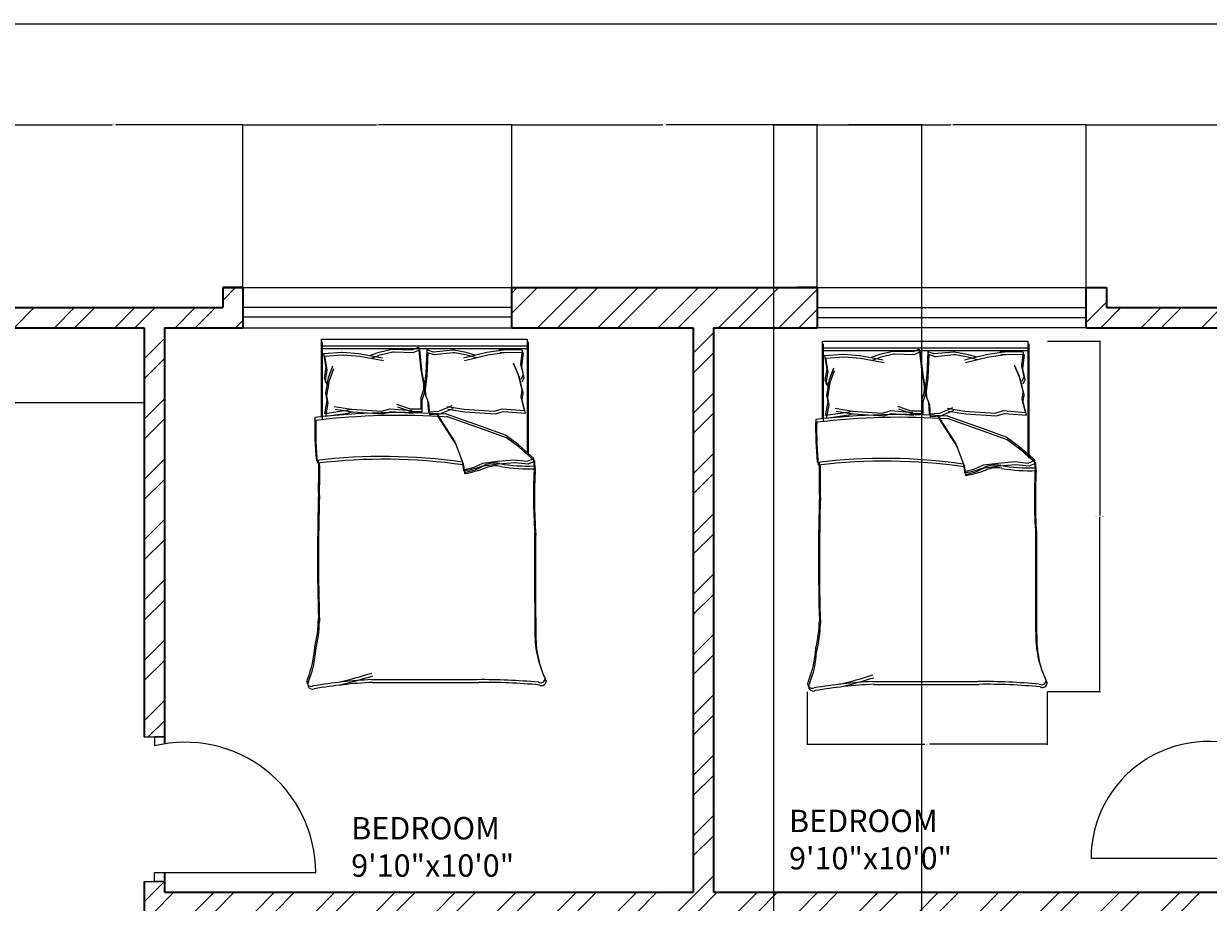
# Model space of a CAD drawing. Units: inches. Extents: x 1570 to 2186, y 1575 to 2421.
# Tile 9 of 10: x 1713 to 1978, y 2225 to 2421. Entities that reach past the tile are written whole.
import ezdxf

# ---------------------------------------------------------------- set-up
doc = ezdxf.new("R2010")
doc.units = ezdxf.units.IN
for name, color, linetype, lineweight in [('A-ANNO-DIMS', 2, 'Continuous', 18), ('A-ANNO-TTLB', 7, 'Continuous', 25), ('A-AREA-IDEN', 7, 'Continuous', 18), ('A-DOOR', 201, 'Continuous', 18), ('A-FLOR-CASE', 7, 'Continuous', 18), ('A-FURN', 8, 'Continuous', 13), ('A-GLAZ', 150, 'Continuous', 18), ('A-WALL', 7, 'Continuous', 35), ('A-WALL-PATT', 252, 'Continuous', 13)]:
    doc.layers.add(name, color=color, linetype=linetype, lineweight=lineweight)
doc.styles.get("Standard").update_dxf_attribs({"font": 'arial.ttf'})
doc.dimstyles.get("Standard").update_dxf_attribs({"dimtxt": 0.18, "dimasz": 0.18, "dimexe": 0.18, "dimexo": 0.0625, "dimgap": 0.09, "dimtad": 0, "dimtih": 1, "dimtoh": 1, "dimdec": 4, "dimzin": 0, "dimdsep": 46, "dimtxsty": 'Standard', "dimcen": 0.09, "dimadec": 0, "dimazin": 0, "dimtfac": 1, "dimtdec": 4, "dimtofl": 0, "dimtmove": 0, "dimatfit": 3, "dimfxl": 1, "dimtolj": 1, "dimtzin": 0, "dimarcsym": 0})

# ---------------------------------------------------------------- blocks, each defined once
blk = doc.blocks.new('BED-DOUBLE')
for p, q in [((3.33, 60.74), (3.33, 78.1)), ((3.33, 60.74), (3.33, 78.1)), ((3.33, 78.1), (49.16, 78.1)), ((3.55, 60.12), (3.55, 77.49)), ((3.55, 60.12), (3.55, 77.49)), ((49.16, 78.1), (49.16, 52.58)), ((49.16, 78.1), (49.16, 52.58)), ((49.38, 77.49), (49.38, 51.97)), ((49.38, 77.49), (49.38, 51.97)), ((3.33, 76.63), (49.16, 76.63)), ((3.33, 76.63), (49.16, 76.63)), ((3.55, 76.02), (49.38, 76.02)), ((3.55, 76.02), (49.38, 76.02)), ((3.74, 74.9), (7.84, 75.22)), ((3.74, 74.9), (7.84, 75.22)), ((3.74, 74.92), (4.29, 71.87)), ((3.74, 74.92), (4.29, 71.87)), ((3.95, 74.31), (4.51, 71.26)), ((3.95, 74.31), (4.51, 71.26)), ((3.96, 74.29), (8.06, 74.6)), ((3.96, 74.29), (8.06, 74.6)), ((7.84, 75.22), (7.95, 75.2)), ((7.84, 75.22), (7.95, 75.2)), ((7.95, 75.2), (11.61, 74.92)), ((7.95, 75.2), (11.61, 74.92)), ((8.06, 74.6), (8.16, 74.59)), ((8.06, 74.6), (8.16, 74.59)), ((8.16, 74.59), (11.83, 74.31)), ((8.16, 74.59), (11.83, 74.31)), ((11.61, 74.92), (16.88, 73.95)), ((11.61, 74.92), (16.88, 73.95)), ((11.83, 74.31), (17.1, 73.34)), ((11.83, 74.31), (17.1, 73.34)), ((14.25, 74.51), (16.19, 75.2)), ((14.25, 74.51), (16.19, 75.2)), ((14.46, 73.89), (16.41, 74.59)), ((14.47, 73.89), (16.41, 74.59)), ((16.19, 75.2), (18.96, 75.89)), ((16.19, 75.2), (18.96, 75.89)), ((16.41, 74.59), (19.18, 75.28)), ((16.41, 74.59), (19.18, 75.28)), ((18.96, 75.89), (19.27, 75.89)), ((18.96, 75.89), (19.27, 75.89)), ((19.18, 75.28), (19.49, 75.28)), ((19.18, 75.28), (19.49, 75.28)), ((19.27, 75.89), (23.53, 75.76)), ((19.27, 75.89), (23.53, 75.76)), ((19.49, 75.28), (23.75, 75.14)), ((19.49, 75.28), (23.75, 75.14)), ((23.53, 75.76), (24.92, 76.31)), ((23.53, 75.76), (24.92, 76.31)), ((23.75, 75.14), (25.14, 75.7)), ((23.75, 75.14), (25.14, 75.7)), ((24.92, 76.31), (25.47, 71.18)), ((24.92, 76.31), (25.47, 71.18)), ((25.14, 75.7), (25.69, 70.57)), ((25.14, 75.7), (25.69, 70.57)), ((26.83, 75.71), (26.6, 70.56)), ((26.83, 75.71), (26.6, 70.56)), ((27.05, 75.1), (26.82, 69.95)), ((27.05, 75.1), (26.82, 69.95)), ((28.25, 75.25), (26.83, 75.71)), ((28.25, 75.25), (26.83, 75.71)), ((28.47, 74.63), (27.05, 75.1)), ((28.47, 74.63), (27.05, 75.1)), ((32.49, 75.65), (28.25, 75.25)), ((32.49, 75.65), (28.25, 75.25)), ((32.71, 75.04), (28.47, 74.63)), ((32.71, 75.04), (28.47, 74.63)), ((32.8, 75.67), (32.49, 75.65)), ((32.8, 75.67), (32.49, 75.65)), ((33.02, 75.06), (32.71, 75.04)), ((33.02, 75.06), (32.71, 75.04)), ((35.61, 75.15), (32.8, 75.67)), ((35.61, 75.15), (32.8, 75.67)), ((35.83, 74.54), (33.02, 75.06)), ((35.83, 74.54), (33.02, 75.06)), ((40.2, 75.16), (35, 73.86)), ((40.2, 75.16), (35, 73.86)), ((40.42, 74.55), (35.22, 73.25)), ((40.41, 74.55), (35.22, 73.25)), ((37.59, 74.58), (35.61, 75.15)), ((37.59, 74.58), (35.61, 75.15)), ((37.81, 73.97), (35.83, 74.54)), ((37.81, 73.97), (35.83, 74.54)), ((43.84, 75.67), (40.2, 75.16)), ((43.84, 75.67), (40.2, 75.16)), ((44.06, 75.05), (40.41, 74.55)), ((44.06, 75.05), (40.42, 74.55)), ((48.06, 75.65), (42.88, 75.74)), ((42.88, 75.74), (43.84, 75.67)), ((48.06, 75.65), (42.88, 75.74)), ((42.88, 75.74), (43.84, 75.67)), ((48.28, 75.04), (43.1, 75.13)), ((43.1, 75.13), (44.06, 75.05)), ((48.28, 75.04), (43.1, 75.13)), ((43.1, 75.13), (44.06, 75.05)), ((48.06, 75.65), (47.69, 72.57)), ((48.06, 75.65), (47.69, 72.57)), ((48.28, 75.04), (47.91, 71.96)), ((48.28, 75.04), (47.91, 71.96)), ((4.29, 71.87), (3.87, 69.38)), ((4.29, 71.87), (3.87, 69.38)), ((4.84, 69.52), (5.81, 72.15)), ((4.84, 69.52), (5.81, 72.15)), ((5.06, 68.9), (6.03, 71.54)), ((5.06, 68.9), (6.03, 71.54)), ((47.29, 70.18), (46.15, 72.75)), ((47.29, 70.18), (46.16, 72.75)), ((47.51, 69.57), (46.37, 72.14)), ((47.51, 69.57), (46.37, 72.14)), ((47.69, 72.57), (48.27, 70.11)), ((47.69, 72.57), (48.26, 70.11)), ((47.91, 71.96), (48.48, 69.49)), ((47.91, 71.96), (48.48, 69.49)), ((3.87, 69.38), (4.43, 68.41)), ((3.87, 69.38), (4.43, 68.41)), ((4.51, 71.26), (4.09, 68.76)), ((4.51, 71.26), (4.09, 68.76)), ((4.09, 68.76), (4.65, 67.79)), ((4.09, 68.76), (4.65, 67.79)), ((4.29, 66.05), (4.84, 69.52)), ((4.29, 66.05), (4.84, 69.52)), ((4.51, 65.44), (5.06, 68.9)), ((4.51, 65.44), (5.06, 68.9)), ((25.47, 71.18), (26.03, 68.13)), ((25.47, 71.18), (26.03, 68.13)), ((25.69, 70.57), (26.25, 67.52)), ((25.69, 70.57), (26.25, 67.52)), ((26.6, 70.56), (26.23, 67.48)), ((26.6, 70.56), (26.23, 67.48)), ((26.82, 69.95), (26.45, 66.87)), ((26.82, 69.95), (26.45, 66.87)), ((48.06, 66.76), (47.29, 70.18)), ((48.06, 66.76), (47.29, 70.18)), ((48.28, 66.15), (47.51, 69.57)), ((48.28, 66.15), (47.51, 69.57)), ((48.27, 70.11), (47.77, 69.1)), ((48.26, 70.11), (47.77, 69.1)), ((48.48, 69.49), (47.99, 68.49)), ((48.48, 69.49), (47.99, 68.49)), ((26.03, 66.88), (25.47, 65.08)), ((26.03, 66.88), (25.47, 65.08)), ((26.25, 66.27), (25.69, 64.47)), ((26.25, 66.27), (25.69, 64.47)), ((26.03, 68.13), (26.03, 66.88)), ((26.03, 68.13), (26.03, 66.88)), ((26.23, 67.48), (26.31, 66.23)), ((26.23, 67.48), (26.31, 66.23)), ((26.25, 67.52), (26.25, 66.27)), ((26.25, 67.52), (26.25, 66.27)), ((26.31, 66.23), (26.98, 64.47)), ((26.31, 66.23), (26.98, 64.47)), ((26.45, 66.87), (26.53, 65.62)), ((26.45, 66.87), (26.53, 65.62)), ((47.88, 65.22), (48.06, 66.76)), ((47.88, 65.22), (48.06, 66.76)), ((48.09, 64.61), (48.28, 66.15)), ((48.1, 64.61), (48.28, 66.15)), ((4.01, 61.47), (4.57, 64.52)), ((4.01, 61.47), (4.57, 64.52)), ((4.23, 60.86), (4.79, 63.91)), ((4.23, 60.86), (4.79, 63.91)), ((4.57, 64.52), (4.29, 66.05)), ((4.57, 64.52), (4.29, 66.05)), ((4.79, 63.91), (4.51, 65.44)), ((4.79, 63.91), (4.51, 65.44)), ((23.12, 62.51), (20.1, 63.55)), ((23.12, 62.51), (20.1, 63.55)), ((25.47, 65.08), (25.47, 62.51)), ((25.47, 65.08), (25.47, 62.51)), ((25.69, 64.47), (25.69, 61.89)), ((25.69, 64.47), (25.69, 61.89)), ((26.53, 65.62), (27.2, 63.86)), ((26.53, 65.62), (27.2, 63.86)), ((26.98, 64.47), (27.14, 61.9)), ((26.98, 64.47), (27.14, 61.9)), ((27.2, 63.86), (27.36, 61.29)), ((27.2, 63.86), (27.36, 61.29)), ((48.62, 62.21), (47.88, 65.22)), ((48.62, 62.21), (47.88, 65.22)), ((48.84, 61.6), (48.09, 64.61)), ((48.84, 61.6), (48.1, 64.61)), ((8.9, 62.17), (4.01, 61.47)), ((8.9, 62.17), (4.01, 61.47)), ((9.12, 61.55), (4.23, 60.86)), ((9.12, 61.55), (4.23, 60.86)), ((6.12, 63.12), (9.99, 62.48)), ((6.12, 63.12), (9.99, 62.48)), ((6.34, 62.5), (10.21, 61.86)), ((6.34, 62.5), (10.21, 61.86)), ((9.99, 62.48), (8.9, 62.17)), ((9.99, 62.48), (8.9, 62.17)), ((10.21, 61.86), (9.12, 61.55)), ((10.21, 61.86), (9.12, 61.55)), ((9.99, 62.48), (16.71, 62.06)), ((9.99, 62.48), (16.71, 62.06)), ((10.21, 61.86), (16.93, 61.45)), ((10.21, 61.86), (16.93, 61.45)), ((16.71, 62.06), (18.59, 62.6)), ((16.71, 62.06), (18.59, 62.6)), ((16.93, 61.45), (18.81, 61.98)), ((16.93, 61.45), (18.81, 61.98)), ((18.59, 62.6), (23.51, 62.21)), ((18.59, 62.6), (23.51, 62.21)), ((18.81, 61.98), (23.73, 61.6)), ((18.81, 61.98), (23.73, 61.6)), ((23.33, 61.89), (20.32, 62.94)), ((23.33, 61.89), (20.32, 62.94)), ((25.47, 62.51), (23.12, 62.51)), ((25.47, 62.51), (23.12, 62.51)), ((25.69, 61.89), (23.33, 61.89)), ((25.69, 61.89), (23.33, 61.89)), ((27.14, 61.9), (29.49, 62.05)), ((27.14, 61.9), (29.49, 62.05)), ((27.36, 61.29), (29.71, 61.44)), ((27.36, 61.29), (29.71, 61.44)), ((29.02, 61.43), (33.04, 55.21)), ((29.02, 61.43), (33.04, 55.21)), ((29.24, 60.82), (33.26, 54.59)), ((29.24, 60.82), (33.26, 54.59)), ((29.49, 62.05), (32.43, 63.28)), ((29.49, 62.05), (32.43, 63.28)), ((29.71, 61.44), (32.65, 62.67)), ((29.71, 61.44), (32.65, 62.67)), ((38.98, 58.62), (30.98, 61.43)), ((38.98, 58.62), (30.98, 61.43)), ((39.2, 58.01), (31.2, 60.82)), ((39.2, 58.01), (31.2, 60.82)), ((31.23, 63.12), (35.1, 62.48)), ((31.23, 63.12), (35.1, 62.48)), ((31.45, 62.5), (35.31, 61.86)), ((31.45, 62.5), (35.31, 61.86)), ((35.1, 62.48), (41.82, 62.06)), ((35.1, 62.48), (41.82, 62.06)), ((35.31, 61.86), (42.04, 61.45)), ((35.31, 61.86), (42.04, 61.45)), ((41.82, 62.06), (43.7, 62.6)), ((41.82, 62.06), (43.7, 62.6)), ((42.04, 61.45), (43.92, 61.98)), ((42.04, 61.45), (43.92, 61.98)), ((43.7, 62.6), (48.62, 62.21)), ((43.7, 62.6), (48.62, 62.21)), ((43.92, 61.98), (48.84, 61.6)), ((43.92, 61.98), (48.84, 61.6)), ((44.32, 56.69), (38.98, 58.62)), ((44.32, 56.69), (38.98, 58.62)), ((44.54, 56.08), (39.2, 58.01)), ((44.54, 56.08), (39.2, 58.01)), ((47.15, 54.61), (44.32, 56.69)), ((47.15, 54.61), (44.32, 56.69)), ((47.37, 54), (44.54, 56.08)), ((47.37, 54), (44.54, 56.08)), ((33.04, 55.21), (34.67, 50.9)), ((33.04, 55.21), (34.67, 50.9)), ((33.26, 54.59), (34.89, 50.29)), ((33.26, 54.59), (34.89, 50.29)), ((50.7, 51.5), (47.15, 54.61)), ((50.7, 51.5), (47.15, 54.61)), ((50.92, 50.88), (47.37, 54)), ((50.92, 50.88), (47.37, 54)), ((34.67, 50.9), (34.97, 48.97)), ((34.67, 50.9), (34.97, 48.97)), ((34.89, 50.29), (35.19, 48.36)), ((34.89, 50.29), (35.19, 48.36)), ((37.34, 49.57), (39.27, 50.46)), ((37.34, 49.57), (39.27, 50.46)), ((39.27, 50.46), (42.54, 50.9)), ((39.27, 50.46), (42.54, 50.9)), ((39.49, 49.84), (42.76, 50.29)), ((39.49, 49.84), (42.76, 50.29)), ((42.54, 50.9), (46.26, 51.2)), ((42.54, 50.9), (46.26, 51.2)), ((42.76, 50.29), (46.47, 50.59)), ((42.76, 50.29), (46.47, 50.59)), ((46.26, 51.2), (49.23, 50.9)), ((46.26, 51.2), (49.23, 50.9)), ((46.47, 50.59), (49.45, 50.29)), ((46.47, 50.59), (49.44, 50.29)), ((49.23, 50.9), (50.7, 51.5)), ((49.23, 50.9), (50.7, 51.5)), ((49.44, 50.29), (50.92, 50.88)), ((49.45, 50.29), (50.92, 50.88)), ((50.78, 49.82), (50.7, 51.5, 3.71)), ((50.78, 49.82), (50.7, 51.5, 3.71)), ((51, 49.21), (50.92, 50.88, 3.71)), ((51, 49.21), (50.92, 50.88, 3.71)), ((34.97, 48.97), (37.34, 49.57)), ((34.97, 48.97), (37.34, 49.57)), ((35.19, 48.36), (37.56, 48.95)), ((35.19, 48.36), (37.56, 48.95)), ((37.56, 48.95), (39.49, 49.84)), ((37.56, 48.95), (39.49, 49.84)), ((14.45, 2.11), (38.05, 2.11)), ((14.45, 2.11), (38.05, 2.11)), ((14.66, 1.49), (38.27, 1.49)), ((14.67, 1.49), (38.27, 1.49))]:
    blk.add_line(p, q)
for centre, radius, start, end in [((20.48, -96.48), 158.2, 86.0865, 96.7821), ((20.48, -96.48), 158.2, 86.0865, 96.7821), ((20.7, -97.1), 158.2, 86.0865, 96.7821), ((20.7, -97.1), 158.2, 86.0865, 96.7821), ((81.67, 58.83), 79.89, 178.7218, 185.604), ((81.67, 58.83), 79.89, 178.7218, 185.604), ((81.89, 58.22), 79.89, 178.7218, 185.604), ((81.89, 58.22), 79.89, 178.7218, 185.604), ((17.03, -71.8), 123.73, 81.7845, 96.9006), ((17.03, -71.8), 123.73, 81.7845, 96.9006), ((17.25, -72.42), 123.73, 81.7845, 96.9006), ((17.25, -72.42), 123.73, 81.7845, 96.9006), ((-160.45, 48.21), 163.13, 358.4762, 1.0082), ((-160.45, 48.21), 163.13, 358.4762, 1.0082), ((-160.23, 47.59), 163.13, 358.4762, 1.0082), ((-160.23, 47.59), 163.13, 358.4762, 1.0082), ((41.95, 44.48), 5.97, 78.6608, 113.7384), ((41.95, 44.48), 5.97, 78.6608, 113.7384), ((49.22, 84.49), 34.7, 259.8763, 272.5657), ((49.22, 84.49), 34.7, 259.8763, 272.5657), ((35.13, 48.91), 0.177, 160.2464, 271.1377), ((35.13, 48.91), 0.177, 160.2464, 271.1377), ((29.88, 76.68), 28.44, 280.6617, 289.8806), ((29.88, 76.68), 28.44, 280.6617, 289.8806), ((35.35, 48.3), 0.177, 160.2464, 271.1377), ((35.35, 48.3), 0.177, 160.2464, 271.1377), ((30.1, 76.07), 28.44, 280.6617, 289.8806), ((30.1, 76.07), 28.44, 280.6617, 289.8806), ((42.17, 43.86), 5.97, 78.6608, 113.7384), ((42.17, 43.86), 5.97, 78.6608, 113.7384), ((49.44, 83.87), 34.7, 259.8763, 272.5657), ((49.44, 83.87), 34.7, 259.8763, 272.5657), ((174.79, 43.28), 124.19, 176.9791, 183.8365), ((174.79, 43.28), 124.19, 176.9791, 183.8365), ((175.01, 42.66), 124.19, 176.9791, 183.8365), ((175.01, 42.66), 124.19, 176.9791, 183.8365), ((464.94, 29.56), 462.53, 178.2277, 181.7185), ((464.94, 29.56), 462.53, 178.2277, 181.7185), ((465.16, 28.95), 462.53, 178.2277, 181.7185), ((465.16, 28.95), 462.53, 178.2277, 181.7185), ((-4323.86, 13.06), 4374.8, 0.00217, 0.28689), ((-4323.86, 13.06), 4374.8, 0.00217, 0.28689), ((-4323.64, 12.45), 4374.8, 0.00217, 0.28689), ((-4323.64, 12.45), 4374.8, 0.00217, 0.28689), ((-25.8, 16.23), 28.42, 346.0648, 358.9113), ((-25.8, 16.23), 28.42, 346.0648, 358.9113), ((-25.58, 15.62), 28.42, 346.0648, 358.9113), ((-25.58, 15.62), 28.42, 346.0648, 358.9113), ((73.03, 12.25), 22.12, 177.4714, 206.4681), ((73.03, 12.25), 22.12, 177.4714, 206.4681), ((73.25, 11.64), 22.12, 177.4714, 206.4681), ((73.25, 11.64), 22.12, 177.4714, 206.4681), ((-20.77, 10.71), 22.6, 337.9751, 356.652), ((-20.77, 10.71), 22.6, 337.9751, 356.652), ((-20.55, 10.1), 22.6, 337.9751, 356.652), ((-20.55, 10.1), 22.6, 337.9751, 356.652), ((-16.52, 100.84), 102.09, 283.3832, 287.7053), ((-16.52, 100.84), 102.09, 283.3832, 287.7053), ((-16.3, 100.23), 102.09, 283.3832, 287.7053), ((-16.3, 100.23), 102.09, 283.3832, 287.7053), ((1.04, 1.65), 1.04, 146.1736, 293.4781), ((1.04, 1.65), 1.04, 146.1736, 293.4781), ((1.26, 1.04), 1.04, 146.1736, 293.4781), ((1.26, 1.04), 1.04, 146.1736, 293.4781), ((20.55, -114.5), 116.77, 92.9958, 99.4091), ((20.55, -114.5), 116.77, 92.9958, 99.4091), ((20.77, -115.11), 116.77, 92.9958, 99.4091), ((20.77, -115.11), 116.77, 92.9958, 99.4091), ((39.46, -125.47), 127.58, 84.4998, 90.6351), ((39.46, -125.47), 127.58, 84.4998, 90.6351), ((39.68, -126.08), 127.58, 84.4998, 90.6351), ((39.68, -126.08), 127.58, 84.4998, 90.6351), ((52.18, 2.47), 1.06, 242.6588, 356.02), ((52.18, 2.47), 1.06, 242.6588, 356.02), ((52.4, 1.85), 1.06, 242.6588, 356.02), ((52.4, 1.85), 1.06, 242.6588, 356.02)]:
    blk.add_arc(centre, radius, start, end)
blk = doc.blocks.new('*D14')
at = {"layer": 'A-ANNO-DIMS', "color": 0, "lineweight": -2, "transparency": 16777216}
for p, q in [((1941.63, 2350.17), (1953.47, 2350.17)), ((1953.29, 2349.99), (1953.29, 2311.25)), ((1953.29, 2272.15), (1953.29, 2310.89)), ((1941.63, 2271.97), (1953.47, 2271.97))]:
    blk.add_line(p, q, dxfattribs=at)
at = {"layer": 'A-ANNO-DIMS', "color": 0, "transparency": 16777216}
for points in [[(1953.26, 2349.99), (1953.32, 2349.99), (1953.29, 2350.17)], [(1953.26, 2272.15), (1953.32, 2272.15), (1953.29, 2271.97)]]:
    blk.add_solid(points, dxfattribs=at)
at = {"layer": 'Defpoints', "color": 0, "transparency": 16777216}
for p in [(1941.56, 2350.17), (1953.29, 2350.17), (1941.56, 2271.97)]:
    blk.add_point(p, dxfattribs=at)
at = {"layer": 'A-ANNO-DIMS', "color": 0, "transparency": 16777216, "insert": (1953.29, 2311.07), "char_height": 0.18, "attachment_point": 5}
blk.add_mtext('\\A1;DOUBLE BED 78 TYP.', dxfattribs=at)
blk = doc.blocks.new('*D15')
at = {"layer": 'A-ANNO-DIMS', "color": 0, "lineweight": -2, "transparency": 16777216}
for p, q in [((1888.03, 2271.91), (1888.03, 2260.06)), ((1941.56, 2271.91), (1941.56, 2260.06)), ((1888.21, 2260.24), (1914.27, 2260.24)), ((1941.38, 2260.24), (1915.32, 2260.24))]:
    blk.add_line(p, q, dxfattribs=at)
at = {"layer": 'A-ANNO-DIMS', "color": 0, "transparency": 16777216}
for points in [[(1888.21, 2260.27), (1888.21, 2260.21), (1888.03, 2260.24)], [(1941.38, 2260.27), (1941.38, 2260.21), (1941.56, 2260.24)]]:
    blk.add_solid(points, dxfattribs=at)
at = {"layer": 'Defpoints', "color": 0, "transparency": 16777216}
for p in [(1888.03, 2271.97), (1941.56, 2271.97), (1941.56, 2260.24)]:
    blk.add_point(p, dxfattribs=at)
at = {"layer": 'A-ANNO-DIMS', "color": 0, "transparency": 16777216, "insert": (1914.8, 2260.24), "char_height": 0.18, "attachment_point": 5}
blk.add_mtext('\\A1;54 TYP.', dxfattribs=at)
blk = doc.blocks.new('*D24')
at = {"layer": 'A-ANNO-DIMS', "color": 0, "lineweight": -2, "transparency": 16777216}
for p, q in [((1704.62, 2362.21), (1704.62, 2398.63)), ((1704.8, 2398.45), (1732.96, 2398.45)), ((1761.92, 2398.45), (1733.75, 2398.45)), ((1762.1, 2362.21), (1762.1, 2398.63))]:
    blk.add_line(p, q, dxfattribs=at)
at = {"layer": 'A-ANNO-DIMS', "color": 0, "transparency": 16777216}
for points in [[(1704.8, 2398.48), (1704.8, 2398.42), (1704.62, 2398.45)], [(1761.92, 2398.48), (1761.92, 2398.42), (1762.1, 2398.45)]]:
    blk.add_solid(points, dxfattribs=at)
at = {"layer": 'Defpoints', "color": 0, "transparency": 16777216}
for p in [(1762.1, 2398.45), (1704.62, 2362.15), (1762.1, 2362.15)]:
    blk.add_point(p, dxfattribs=at)
at = {"layer": 'A-ANNO-DIMS', "color": 0, "transparency": 16777216, "insert": (1733.36, 2398.45), "char_height": 0.18, "attachment_point": 5}
blk.add_mtext('\\A1;57.48', dxfattribs=at)
blk = doc.blocks.new('*D25')
at = {"layer": 'A-ANNO-DIMS', "color": 0, "lineweight": -2, "transparency": 16777216}
for p, q in [((1762.1, 2362.21), (1762.1, 2398.63)), ((1762.28, 2398.45), (1791.88, 2398.45)), ((1821.92, 2398.45), (1792.32, 2398.45)), ((1822.1, 2362.21), (1822.1, 2398.63))]:
    blk.add_line(p, q, dxfattribs=at)
at = {"layer": 'A-ANNO-DIMS', "color": 0, "transparency": 16777216}
for points in [[(1762.28, 2398.48), (1762.28, 2398.42), (1762.1, 2398.45)], [(1821.92, 2398.48), (1821.92, 2398.42), (1822.1, 2398.45)]]:
    blk.add_solid(points, dxfattribs=at)
at = {"layer": 'Defpoints', "color": 0, "transparency": 16777216}
for p in [(1822.1, 2398.45), (1762.1, 2362.15), (1822.1, 2362.15)]:
    blk.add_point(p, dxfattribs=at)
at = {"layer": 'A-ANNO-DIMS', "color": 0, "transparency": 16777216, "insert": (1792.1, 2398.45), "char_height": 0.18, "attachment_point": 5}
blk.add_mtext('\\A1;60', dxfattribs=at)
blk = doc.blocks.new('*D26')
at = {"layer": 'A-ANNO-DIMS', "color": 0, "lineweight": -2, "transparency": 16777216}
for p, q in [((1822.1, 2362.21), (1822.1, 2398.63)), ((1822.28, 2398.45), (1855.78, 2398.45)), ((1890.08, 2398.45), (1856.57, 2398.45)), ((1890.26, 2362.21), (1890.26, 2398.63))]:
    blk.add_line(p, q, dxfattribs=at)
at = {"layer": 'A-ANNO-DIMS', "color": 0, "transparency": 16777216}
for points in [[(1822.28, 2398.48), (1822.28, 2398.42), (1822.1, 2398.45)], [(1890.08, 2398.48), (1890.08, 2398.42), (1890.26, 2398.45)]]:
    blk.add_solid(points, dxfattribs=at)
at = {"layer": 'Defpoints', "color": 0, "transparency": 16777216}
for p in [(1890.26, 2398.45), (1822.1, 2362.15), (1890.26, 2362.15)]:
    blk.add_point(p, dxfattribs=at)
at = {"layer": 'A-ANNO-DIMS', "color": 0, "transparency": 16777216, "insert": (1856.18, 2398.45), "char_height": 0.18, "attachment_point": 5}
blk.add_mtext('\\A1;68.16', dxfattribs=at)
blk = doc.blocks.new('*D27')
at = {"layer": 'A-ANNO-DIMS', "color": 0, "lineweight": -2, "transparency": 16777216}
for p, q in [((1890.26, 2362.21), (1890.26, 2398.63)), ((1890.44, 2398.45), (1920.04, 2398.45)), ((1950.08, 2398.45), (1920.48, 2398.45)), ((1950.26, 2362.21), (1950.26, 2398.63))]:
    blk.add_line(p, q, dxfattribs=at)
at = {"layer": 'A-ANNO-DIMS', "color": 0, "transparency": 16777216}
for points in [[(1890.44, 2398.48), (1890.44, 2398.42), (1890.26, 2398.45)], [(1950.08, 2398.48), (1950.08, 2398.42), (1950.26, 2398.45)]]:
    blk.add_solid(points, dxfattribs=at)
at = {"layer": 'Defpoints', "color": 0, "transparency": 16777216}
for p in [(1950.26, 2398.45), (1890.26, 2362.15), (1950.26, 2362.15)]:
    blk.add_point(p, dxfattribs=at)
at = {"layer": 'A-ANNO-DIMS', "color": 0, "transparency": 16777216, "insert": (1920.26, 2398.45), "char_height": 0.18, "attachment_point": 5}
blk.add_mtext('\\A1;60', dxfattribs=at)
blk = doc.blocks.new('*D28')
at = {"layer": 'A-ANNO-DIMS', "color": 0, "lineweight": -2, "transparency": 16777216}
for p, q in [((1950.26, 2362.21), (1950.26, 2398.63)), ((1950.44, 2398.45), (1981.26, 2398.45)), ((2012.86, 2398.45), (1982.05, 2398.45)), ((2013.04, 2362.21), (2013.04, 2398.63))]:
    blk.add_line(p, q, dxfattribs=at)
at = {"layer": 'A-ANNO-DIMS', "color": 0, "transparency": 16777216}
for points in [[(1950.44, 2398.48), (1950.44, 2398.42), (1950.26, 2398.45)], [(2012.86, 2398.48), (2012.86, 2398.42), (2013.04, 2398.45)]]:
    blk.add_solid(points, dxfattribs=at)
at = {"layer": 'Defpoints', "color": 0, "transparency": 16777216}
for p in [(2013.04, 2398.45), (1950.26, 2362.15), (2013.04, 2362.15)]:
    blk.add_point(p, dxfattribs=at)
at = {"layer": 'A-ANNO-DIMS', "color": 0, "transparency": 16777216, "insert": (1981.65, 2398.45), "char_height": 0.18, "attachment_point": 5}
blk.add_mtext('\\A1;62.78', dxfattribs=at)
blk = doc.blocks.new('*D45')
at = {"layer": 'A-ANNO-DIMS', "color": 0, "lineweight": -2, "transparency": 16777216}
for p, q in [((1880.59, 1913.81), (1880.59, 2398.63)), ((1880.77, 2398.45), (1896.87, 2398.45)), ((1913.41, 2398.45), (1897.31, 2398.45)), ((1913.59, 1913.81), (1913.59, 2398.63))]:
    blk.add_line(p, q, dxfattribs=at)
at = {"layer": 'A-ANNO-DIMS', "color": 0, "transparency": 16777216}
for points in [[(1880.77, 2398.48), (1880.77, 2398.42), (1880.59, 2398.45)], [(1913.41, 2398.48), (1913.41, 2398.42), (1913.59, 2398.45)]]:
    blk.add_solid(points, dxfattribs=at)
at = {"layer": 'Defpoints', "color": 0, "transparency": 16777216}
for p in [(1913.59, 2398.45), (1880.59, 1913.75), (1913.59, 1913.75)]:
    blk.add_point(p, dxfattribs=at)
at = {"layer": 'A-ANNO-DIMS', "color": 0, "transparency": 16777216, "insert": (1897.09, 2398.45), "char_height": 0.18, "attachment_point": 5}
blk.add_mtext('\\A1;33', dxfattribs=at)

msp = doc.modelspace()

# ---------------------------------------------------------------- hatches: boundary and pattern name
at = {"layer": 'A-WALL-PATT'}
h = msp.add_hatch(dxfattribs=at)
h.set_pattern_fill('ANSI32', color=256)
h.paths.add_polyline_path([(1762.0975, 2362.1492), (1757.5975, 2362.1492), (1757.5975, 2357.6492), (1709.1163, 2357.6492), (1709.1163, 2362.1492), (1704.6163, 2362.1492), (1704.6163, 2353.1492), (1740.0886, 2353.1492), (1740.0886, 2261.8115), (1744.5886, 2261.8115), (1744.5886, 2353.1492), (1762.0975, 2353.1492)])
h.paths.add_polyline_path([(1890.2592, 2362.1492), (1885.7592, 2362.1492), (1826.5975, 2362.1492), (1822.0975, 2362.1492), (1822.0975, 2353.1492), (1862.5886, 2353.1492), (1862.5886, 2227.1492), (1744.5886, 2227.1492), (1744.5886, 2229.5389), (1742.3386, 2229.5389), (1740.0886, 2229.5389), (1740.0886, 2222.6492), (1744.5886, 2222.6492), (1756.186, 2222.6492), (1756.186, 2216.3571), (1760.686, 2216.3571), (1760.686, 2222.6492), (1832.686, 2222.6492), (1832.686, 2212.5994), (1837.186, 2212.5994), (1837.186, 2222.6492), (1893.186, 2222.6492), (1893.186, 2212.5994), (1897.686, 2212.5994), (1897.686, 2222.6492), (1989.5886, 2222.6492), (1989.5886, 2227.1492), (1989.5886, 2232.6585), (1987.3386, 2232.6585), (1985.0886, 2232.6585), (1985.0886, 2227.1492), (1867.0886, 2227.1492), (1867.0886, 2353.1492), (1890.2592, 2353.1492)])
h.paths.add_polyline_path([(1644.0886, 2353.1492), (1668.6163, 2353.1492), (1668.6163, 2362.1492), (1664.1163, 2362.1492), (1664.1163, 2358.9932), (1664.1163, 2357.6492), (1639.5886, 2357.6492), (1639.5886, 2213.8746), (1644.0886, 2213.8746), (1644.0886, 2222.6492), (1692.0886, 2222.6492), (1692.0886, 2215.9343), (1696.5886, 2215.9343), (1696.5886, 2222.6492), (1696.5886, 2227.1492), (1644.0886, 2227.1492)])
h.paths.add_polyline_path([(2013.0435, 2362.1492), (2008.5435, 2362.1492), (2008.5435, 2357.6492), (1954.7592, 2357.6492), (1954.7592, 2362.1492), (1950.2592, 2362.1492), (1950.2592, 2353.1492), (1985.0886, 2353.1492), (1985.0886, 2260.8534), (1989.5886, 2260.8534), (1989.5886, 2353.1492), (2013.0435, 2353.1492)])
h.paths.add_polyline_path([(2090.0886, 2357.6492), (2053.5435, 2357.6492), (2053.5435, 2362.1492), (2049.0435, 2362.1492), (2049.0435, 2353.1492), (2085.5886, 2353.1492), (2085.5886, 2227.1492), (2033.0886, 2227.1492), (2033.0886, 2222.6492), (2033.0886, 2214.4464), (2037.5886, 2214.4464), (2037.5886, 2222.6492), (2085.5886, 2222.6492), (2085.5886, 2212.4409), (2090.0886, 2212.4409)])
h.paths.add_polyline_path([(2090.0886, 2188.4409), (2087.8386, 2188.4409), (2085.5886, 2188.4409), (2085.5886, 2180.6492), (2037.5886, 2180.6492), (2037.5886, 2196.7956), (2033.0886, 2196.7956), (2033.0886, 2176.1492), (2037.5886, 2176.1492), (2045.0886, 2176.1492), (2045.0886, 2169.8988), (2049.5886, 2169.8988), (2049.5886, 2176.1492), (2085.5886, 2176.1492), (2085.5886, 2167.785), (2090.0886, 2167.785)])
h.paths.add_polyline_path([(2049.5886, 2147.4502), (2047.3386, 2147.4502), (2045.0886, 2147.4502), (2045.0886, 2124.4703), (2049.5886, 2124.4703)])
h.paths.add_polyline_path([(2090.0886, 2047.1492), (2049.5886, 2047.1492), (2049.5886, 2064.4703), (2045.0886, 2064.4703), (2045.0886, 2047.1492), (1918.0886, 2047.1492), (1918.0886, 2051.2061), (1913.5886, 2051.2061), (1913.5886, 2047.1492), (1913.5886, 2036.6872), (1918.0886, 2036.6872), (1918.0886, 2042.7492), (2045.0886, 2042.7492), (2045.0886, 2027.0686), (2049.5886, 2027.0686), (2049.5886, 2042.7492), (2090.0886, 2042.7492)])
h.paths.add_polyline_path([(1918.0886, 2005.9338), (1915.8386, 2005.9338), (1913.5886, 2005.9338), (1913.5886, 1913.7492), (1918.0886, 1913.7492)])
h.paths.add_polyline_path([(2090.0886, 1913.7492), (2049.5886, 1913.7492), (2045.0886, 1913.7492), (2033.0886, 1913.7492), (2033.0886, 1909.2492), (2033.0886, 1900.9803), (2037.5886, 1900.9803), (2037.5886, 1909.2492), (2085.5886, 1909.2492), (2085.5886, 1861.2492), (2037.5886, 1861.2492), (2037.5886, 1880.0859), (2033.0886, 1880.0859), (2033.0886, 1856.7492), (2085.5886, 1856.7492), (2085.5886, 1730.7492), (2054.2483, 1730.7492), (2054.2483, 1721.7492), (2058.7483, 1721.7492), (2058.7483, 1726.2492), (2090.0886, 1726.2492)])
h.paths.add_polyline_path([(2049.5886, 1967.0686), (2045.0886, 1967.0686), (2045.0886, 1913.7492), (2049.5886, 1913.7492)])
h.paths.add_polyline_path([(1989.5886, 1824.1695), (1987.3386, 1824.1695), (1985.0886, 1824.1695), (1985.0886, 1730.7492), (1989.5886, 1730.7492)])
h.paths.add_polyline_path([(1989.5886, 1861.2492), (1974.9963, 1861.2492), (1974.9963, 1865.9306), (1972.7463, 1865.9306), (1970.4963, 1865.9306), (1970.4963, 1861.2492), (1898.4963, 1861.2492), (1898.4963, 1874.2999), (1893.9963, 1874.2999), (1893.9963, 1861.2492), (1890.5886, 1861.2492), (1837.9963, 1861.2492), (1837.9963, 1874.3159), (1833.4963, 1874.3159), (1833.4963, 1861.2492), (1761.4963, 1861.2492), (1761.4963, 1865.0209), (1759.2463, 1865.0209), (1756.9963, 1865.0209), (1756.9963, 1861.2492), (1740.0886, 1861.2492), (1740.0886, 1856.7492), (1740.0886, 1850.7206), (1744.5886, 1850.7206), (1744.5886, 1856.7492), (1985.0886, 1856.7492), (1985.0886, 1851.0804), (1989.5886, 1851.0804), (1989.5886, 1856.7492)])
h.paths.add_polyline_path([(1989.5886, 1913.7492), (1740.0886, 1913.7492), (1740.0886, 1909.2492), (1756.9963, 1909.2492), (1756.9963, 1890.279), (1761.4963, 1890.279), (1761.4963, 1909.2492), (1833.4963, 1909.2492), (1833.4963, 1898.3159), (1837.9963, 1898.3159), (1837.9963, 1909.2492), (1890.5886, 1909.2492), (1893.9963, 1909.2492), (1893.9963, 1898.2999), (1898.4963, 1898.2999), (1898.4963, 1909.2492), (1970.4963, 1909.2492), (1970.4963, 1886.9887), (1974.9963, 1886.9887), (1974.9963, 1909.2492), (1989.5886, 1909.2492)])
h.paths.add_polyline_path([(1893.7344, 1730.7492), (1867.0886, 1730.7492), (1867.0886, 1856.7492), (1862.5886, 1856.7492), (1862.5886, 1730.7492), (1824.0492, 1730.7492), (1824.0492, 1721.7492), (1893.7344, 1721.7492)])
h.paths.add_polyline_path([(2018.2483, 1730.7492), (1953.7344, 1730.7492), (1953.7344, 1721.7492), (1958.2344, 1721.7492), (1958.2344, 1726.2492), (2013.7483, 1726.2492), (2013.7483, 1721.7492), (2018.2483, 1721.7492)])
h.paths.add_polyline_path([(1768.5492, 1730.7492), (1764.0492, 1730.7492), (1744.5886, 1730.7492), (1744.5886, 1819.4364), (1742.3386, 1819.4364), (1740.0886, 1819.4364), (1740.0886, 1730.7492), (1697.3801, 1730.7492), (1697.3801, 1721.7492), (1701.8801, 1721.7492), (1701.8801, 1726.2492), (1764.0492, 1726.2492), (1764.0492, 1721.7492), (1768.5492, 1721.7492)])
h.paths.add_polyline_path([(1644.0886, 1856.7492), (1639.5886, 1856.7492), (1639.5886, 1726.2492), (1657.0315, 1726.2492), (1657.0315, 1721.7492), (1661.3801, 1721.7492), (1661.3801, 1730.7492), (1644.0886, 1730.7492)])
h.paths.add_polyline_path([(1696.5886, 1876.1809), (1692.0886, 1876.1809), (1692.0886, 1861.2492), (1684.5886, 1861.2492), (1644.0886, 1861.2492), (1644.0886, 1909.2492), (1692.0886, 1909.2492), (1692.0886, 1900.3394), (1696.5886, 1900.3394), (1696.5886, 1913.7492), (1684.5886, 1913.7492), (1684.5886, 1920.2115), (1682.3386, 1920.2115), (1680.0886, 1920.2115), (1680.0886, 1913.7492), (1639.5886, 1913.7492), (1639.5886, 1856.7492), (1684.5886, 1856.7492), (1692.0886, 1856.7492), (1696.5886, 1856.7492)])
h.paths.add_polyline_path([(1684.5886, 2042.7492), (1811.5886, 2042.7492), (1811.5886, 2038.2991), (1816.0886, 2038.2991), (1816.0886, 2042.7492), (1816.0886, 2052.5708), (1813.8386, 2052.5708), (1811.5886, 2052.5708), (1811.5886, 2047.1492), (1684.5886, 2047.1492), (1684.5886, 2064.4703), (1680.0886, 2064.4703), (1680.0886, 2047.1492), (1639.5886, 2047.1492), (1639.5886, 2042.7492), (1680.0886, 2042.7492), (1680.0886, 2024.0762), (1684.5886, 2024.0762)])
h.paths.add_polyline_path([(1684.5886, 1964.0762), (1680.0886, 1964.0762), (1680.0886, 1944.6145), (1684.5886, 1944.6145)])
h.paths.add_polyline_path([(1816.0886, 1973.7492), (1876.0886, 1973.7492), (1876.0886, 1959.17), (1880.5886, 1959.17), (1880.5886, 1973.7492), (1880.5886, 1978.2492), (1816.0886, 1978.2492), (1816.0886, 2005.9338), (1813.8386, 2005.9338), (1811.5886, 2005.9338), (1811.5886, 1913.7492), (1816.0886, 1913.7492)])
h.paths.add_polyline_path([(1837.186, 2180.6492), (1837.186, 2188.5994), (1834.936, 2188.5994), (1832.686, 2188.5994), (1832.686, 2180.6492), (1760.686, 2180.6492), (1760.686, 2197.4807), (1756.186, 2197.4807), (1756.186, 2180.6492), (1744.5886, 2180.6492), (1740.0886, 2180.6492), (1740.0886, 2176.1492), (1837.186, 2176.1492)])
h.paths.add_polyline_path([(1974.186, 2196.8744), (1971.936, 2196.8744), (1969.686, 2196.8744), (1969.686, 2180.6492), (1897.686, 2180.6492), (1897.686, 2188.5994), (1895.436, 2188.5994), (1893.186, 2188.5994), (1893.186, 2180.6492), (1893.186, 2176.1492), (1974.186, 2176.1492)])
h.paths.add_polyline_path([(1918.0886, 2176.1492), (1913.5886, 2176.1492), (1913.5886, 2081.3709), (1918.0886, 2081.3709)])
h.paths.add_polyline_path([(1816.0886, 2176.1492), (1811.5886, 2176.1492), (1811.5886, 2081.3709), (1816.0886, 2081.3709)])
h.paths.add_polyline_path([(1684.5886, 2150.4939), (1682.3386, 2150.4939), (1680.0886, 2150.4939), (1680.0886, 2124.4703), (1684.5886, 2124.4703)])
h.paths.add_polyline_path([(1696.5886, 2180.6492), (1696.5886, 2197.4701), (1692.0886, 2197.4701), (1692.0886, 2180.6492), (1644.0886, 2180.6492), (1644.0886, 2189.8746), (1641.8386, 2189.8746), (1639.5886, 2189.8746), (1639.5886, 2169.814), (1644.0886, 2169.814), (1644.0886, 2176.1492), (1680.0886, 2176.1492), (1680.0886, 2171.7002), (1684.5886, 2171.7002), (1684.5886, 2176.1492), (1696.5886, 2176.1492)])

# ---------------------------------------------------------------- linework, layer by layer
at = {"layer": 'A-ANNO-TTLB'}
msp.add_lwpolyline([(1569.8198, 2421.0436), (2186.3437, 2421.0436), (2186.3437, 1574.5084), (1569.8198, 1574.5084)], close=True, dxfattribs=at)
at = {"layer": 'A-DOOR'}
for p, q in [((1740.0886, 2261.8115), (1744.5886, 2261.8115)), ((1744.5886, 2261.8115), (1742.3386, 2261.8115)), ((1742.3386, 2261.8115), (1742.3386, 2259.8115)), ((1987.3386, 2234.6585), (1951.3386, 2234.6585)), ((1742.3386, 2229.5389), (1742.3386, 2231.5389)), ((1742.3386, 2231.5389), (1778.3386, 2231.5389)), ((1740.0886, 2229.5389), (1744.5886, 2229.5389)), ((1744.5886, 2229.5389), (1742.3386, 2229.5389))]:
    msp.add_line(p, q, dxfattribs=at)
for centre, radius, start, end in [((1749.2366, 2231.5389), 29.102, 0, 103.711244), ((1977.4691, 2234.6585), 26.1305, 67.808551, 180)]:
    msp.add_arc(centre, radius, start, end, dxfattribs=at)
at = {"layer": 'A-FLOR-CASE'}
msp.add_line((1660.2219, 2336.4511), (1740.0886, 2336.4511), dxfattribs=at)
at = {"layer": 'A-GLAZ'}
for p, q in [((1762.0975, 2362.1492), (1824.3475, 2362.1492)), ((1890.2592, 2362.1492), (1950.2592, 2362.1492)), ((1822.0975, 2357.6492), (1762.0975, 2357.6492)), ((1762.0975, 2355.6342), (1822.0975, 2355.6342)), ((1890.2592, 2357.6492), (1950.2592, 2357.6492)), ((1890.2592, 2355.4354), (1950.2592, 2355.4354)), ((1762.0975, 2353.1492), (1822.0975, 2353.1492)), ((1950.2592, 2353.1492), (1890.2592, 2353.1492))]:
    msp.add_line(p, q, dxfattribs=at)
at = {"layer": 'A-WALL'}
for p, q in [((1762.0975, 2362.1492), (1757.5975, 2362.1492)), ((1757.5975, 2362.1492), (1757.5975, 2357.6492)), ((1757.5975, 2362.1492), (1762.0975, 2362.1492)), ((1762.0975, 2362.1492), (1762.0975, 2353.1492)), ((1822.0975, 2353.1492), (1822.0975, 2362.1492)), ((1822.0975, 2362.1492), (1826.5975, 2362.1492)), ((1822.0975, 2362.1492), (1826.5975, 2362.1492)), ((1826.5975, 2362.1492), (1885.7592, 2362.1492)), ((1890.2592, 2362.1492), (1885.7592, 2362.1492)), ((1885.7592, 2362.1492), (1890.2592, 2362.1492)), ((1890.2592, 2362.1492), (1890.2592, 2353.1492)), ((1950.2592, 2353.1492), (1950.2592, 2362.1492)), ((1950.2592, 2362.1492), (1954.7592, 2362.1492)), ((1950.2592, 2362.1492), (1954.7592, 2362.1492)), ((1954.7592, 2362.1492), (1954.7592, 2357.6492)), ((1709.1163, 2357.6492), (1757.5975, 2357.6492)), ((1954.7592, 2357.6492), (2008.5435, 2357.6492)), ((1704.6163, 2353.1492), (1740.0886, 2353.1492)), ((1740.0886, 2353.1492), (1740.0886, 2261.8115)), ((1744.5886, 2353.1492), (1744.5886, 2260.2673)), ((1744.5886, 2353.1492), (1762.0975, 2353.1492)), ((1822.0975, 2353.1492), (1862.5886, 2353.1492)), ((1862.5886, 2353.1492), (1862.5886, 2227.1492)), ((1867.0886, 2353.1492), (1867.0886, 2227.1492)), ((1867.0886, 2353.1492), (1890.2592, 2353.1492)), ((1950.2592, 2353.1492), (1985.0886, 2353.1492)), ((1744.5886, 2231.5389), (1744.5886, 2227.1492)), ((1740.0886, 2229.5389), (1740.0886, 2222.6492)), ((1744.5886, 2227.1492), (1862.5886, 2227.1492)), ((1867.0886, 2227.1492), (1985.0886, 2227.1492))]:
    msp.add_line(p, q, dxfattribs=at)

# ---------------------------------------------------------------- block references
at = {"layer": 'A-FURN'}
for p in [(1776.341, 2272.498), (1888.1104, 2272.0691)]:
    msp.add_blockref('BED-DOUBLE', p, dxfattribs=at)

# ---------------------------------------------------------------- texts
at = {"layer": 'A-AREA-IDEN', "char_height": 5, "attachment_point": 1}
for width, insert in [(115.680291, (1883.9576, 2245.5754)), (130.576826, (1786.2629, 2243.9401))]:
    msp.add_mtext_dynamic_manual_height_columns('BEDROOM\\P9\'10"x10\'0"', width=width, gutter_width=12.5, heights=[0], dxfattribs=dict(at, insert=insert))

# ---------------------------------------------------------------- dimensions: what is measured, and where the dimension line sits
at = {"layer": 'A-ANNO-DIMS'}
for base, p1, p2, override, picture, middle in [((1762.0975, 2398.4492), (1704.6163, 2362.1492), (1762.0975, 2362.1492), {"dimdec": 2, "dimlfac": 1, "dimrnd": 0, "dimzin": 0, "dimdsep": 46, "dimlunit": 2}, '*D24', (1733.3569, 2398.4492)), ((1822.0975, 2398.4492), (1762.0975, 2362.1492), (1822.0975, 2362.1492), {"dimdec": 0, "dimlfac": 1, "dimrnd": 0, "dimzin": 0, "dimdsep": 46, "dimlunit": 2}, '*D25', (1792.0975, 2398.4492)), ((1890.2592, 2398.4492), (1822.0975, 2362.1492), (1890.2592, 2362.1492), {"dimdec": 2, "dimlfac": 1, "dimrnd": 0, "dimzin": 0, "dimdsep": 46, "dimlunit": 2}, '*D26', (1856.1784, 2398.4492)), ((1913.5886, 2398.4492), (1880.5886, 1913.7492), (1913.5886, 1913.7492), {"dimdec": 0, "dimlfac": 1, "dimrnd": 0, "dimzin": 0, "dimdsep": 46, "dimlunit": 2}, '*D45', (1897.0886, 2398.4492)), ((1950.2592, 2398.4492), (1890.2592, 2362.1492), (1950.2592, 2362.1492), {"dimdec": 0, "dimlfac": 1, "dimrnd": 0, "dimzin": 0, "dimdsep": 46, "dimlunit": 2}, '*D27', (1920.2592, 2398.4492)), ((2013.0435, 2398.4492), (1950.2592, 2362.1492), (2013.0435, 2362.1492), {"dimdec": 2, "dimlfac": 1, "dimrnd": 0, "dimzin": 0, "dimdsep": 46, "dimlunit": 2}, '*D28', (1981.6513, 2398.4492))]:
    dim = msp.add_linear_dim(base=base, p1=p1, p2=p2, dimstyle='Standard', override=override, dxfattribs=at)
    dim.commit()
    dim.dimension.update_dxf_attribs({"geometry": picture, "text_midpoint": middle})
dim = msp.add_linear_dim(base=(1953.294, 2350.1725), p1=(1941.5633, 2271.9678), p2=(1941.5633, 2350.1725), angle=90, text='DOUBLE BED <> TYP.', dimstyle='Standard', override={"dimdec": 0, "dimlfac": 1, "dimrnd": 0, "dimzin": 0, "dimdsep": 46, "dimlunit": 2}, dxfattribs=at)
dim.commit()
dim.dimension.update_dxf_attribs({"geometry": '*D14', "text_midpoint": (1953.294, 2311.0702)})
dim = msp.add_linear_dim(base=(1941.5633, 2260.2371), p1=(1888.0278, 2271.9678), p2=(1941.5633, 2271.9678), text='<> TYP.', dimstyle='Standard', override={"dimdec": 0, "dimlfac": 1, "dimrnd": 0, "dimzin": 0, "dimdsep": 46, "dimlunit": 2}, dxfattribs=at)
dim.commit()
dim.dimension.update_dxf_attribs({"geometry": '*D15', "text_midpoint": (1914.7955, 2260.2371)})

doc.saveas('drawing.dxf')
